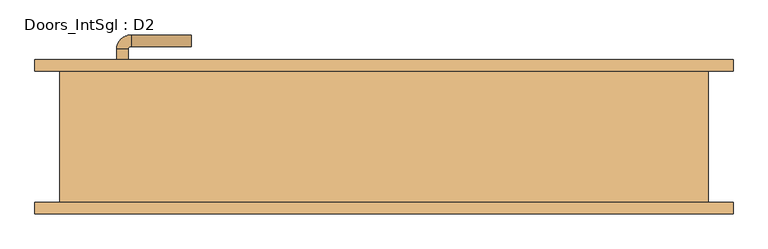
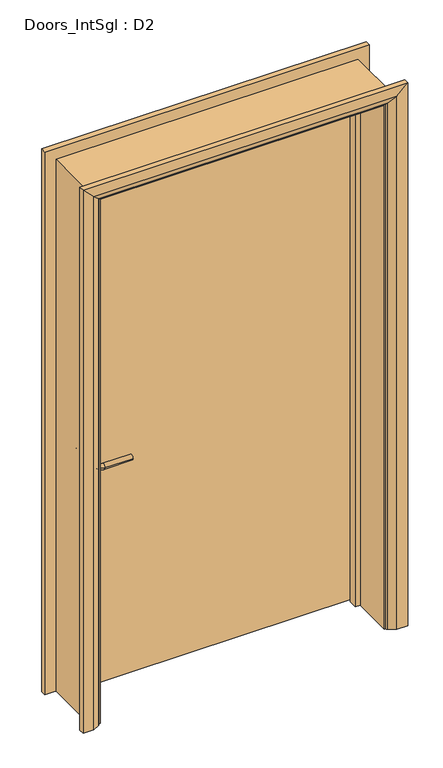
"""IFC4 building model written with IfcOpenShell, lengths in millimetres: door geometry, Doors_IntSgl : D2."""

from ifc_helpers import new_model, si_unit, point, frame, frame_2d, origin, place, context, project, spatial, polyline, circle_curve, ellipse_curve, trimmed, segment, composite_curve, outline, extrude, faceted_brep, source, transform, mapped, element, save
from ifc_brep_helpers import plane_surface, cylinder_surface, revolved_surface, advanced_brep


def doors_intsgl_d2_df50d10e(model_context):
    return source(origin(), model_context, "Body", "SolidModel", [
        advanced_brep(
        [(-464.5, 68.3, 900.0), (-444.5, 68.3, 900.0), (-444.5, 38.3, 900.0), (-464.5, 38.3, 900.0), (-439.5, 33.3, 900.0), (-439.5, 13.3, 900.0), (-334.5, 13.3, 900.0), (-334.5, 33.3, 900.0)],
        [
            (0, 1, circle_curve(frame((-454.5, 68.3, 900.0), z_axis=(0.0, 1.0, 0.0), x_axis=(1.0, 0.0, 0.0)), 10.0)),
            (1, 0, circle_curve(frame((-454.5, 68.3, 900.0), z_axis=(0.0, 1.0, 0.0), x_axis=(1.0, 0.0, 0.0)), 10.0)),
            (1, 2),
            (2, 3, circle_curve(frame((-454.5, 38.3, 900.0), z_axis=(0.0, 1.0, 0.0), x_axis=(1.0, 0.0, 0.0)), 10.0)),
            (3, 0),
            (3, 2, circle_curve(frame((-454.5, 38.3, 900.0), z_axis=(0.0, 1.0, 0.0), x_axis=(1.0, 0.0, 0.0)), 10.0)),
            (4, 5, circle_curve(frame((-439.5, 23.3, 900.0), z_axis=(-1.0, 0.0, 0.0), x_axis=(0.0, 1.0, 0.0)), 10.0)),
            (5, 3, circle_curve(frame((-439.5, 38.3, 900.0), z_axis=(0.0, 0.0, -1.0), x_axis=(-1.0, 0.0, 0.0)), 25.0)),
            (2, 4, circle_curve(frame((-439.5, 38.3, 900.0), z_axis=(0.0, 0.0, 1.0), x_axis=(-1.0, 0.0, 0.0)), 5.0)),
            (5, 4, circle_curve(frame((-439.5, 23.3, 900.0), z_axis=(-1.0, 0.0, 0.0), x_axis=(0.0, 1.0, 0.0)), 10.0)),
            (6, 7, circle_curve(frame((-334.5, 23.3, 900.0), z_axis=(1.0, 0.0, 0.0), x_axis=(0.0, 1.0, 0.0)), 10.0)),
            (7, 6, circle_curve(frame((-334.5, 23.3, 900.0), z_axis=(1.0, 0.0, 0.0), x_axis=(0.0, 1.0, 0.0)), 10.0)),
            (4, 7),
            (6, 5),
        ],
        [
            plane_surface(frame((-454.5, 68.3, 900.0), z_axis=(0.0, 1.0, 0.0), x_axis=(0.0, 0.0, 1.0))),
            cylinder_surface(frame((-454.5, 68.3, 900.0), z_axis=(0.0, 1.0, 0.0), x_axis=(1.0, 0.0, 0.0)), 10.0),
            revolved_surface(trimmed(ellipse_curve(frame((-454.5, 38.3, 900.0), z_axis=(0.0, -1.0, 0.0), x_axis=(1.0, 0.0, 0.0)), 10.0, 10.0), [point((-464.5, 38.3, 900.0))], [point((-444.5, 38.3, 900.0))], True, "CARTESIAN"), (-439.5, 38.3, 900.0), (0.0, 0.0, -1.0)),
            revolved_surface(trimmed(ellipse_curve(frame((-454.5, 38.3, 900.0), z_axis=(0.0, -1.0, 0.0), x_axis=(1.0, 0.0, 0.0)), 10.0, 10.0), [point((-444.5, 38.3, 900.0))], [point((-464.5, 38.3, 900.0))], True, "CARTESIAN"), (-439.5, 38.3, 900.0), (0.0, 0.0, -1.0)),
            plane_surface(frame((-334.5, 23.3, 900.0), z_axis=(1.0, 0.0, 0.0), x_axis=(0.0, 0.0, 1.0))),
            cylinder_surface(frame((-439.5, 23.3, 900.0), z_axis=(-1.0, 0.0, 0.0), x_axis=(0.0, 1.0, 0.0)), 10.0),
        ],
        [
            (0, [[1, 2]]),
            (1, [[3, 4, 5, -2]]),
            (1, [[-5, 6, -3, -1]]),
            (2, [[7, 8, -4, 9]]),
            (3, [[10, -9, -6, -8]]),
            (4, [[11, 12]]),
            (5, [[13, -11, 14, -7]]),
            (5, [[-14, -12, -13, -10]]),
        ],
    ),
        extrude(outline(composite_curve([segment(trimmed(circle_curve(frame_2d((900.0, -457.0)), 30.0), [point((900.0, -487.0))], [point((900.0, -427.0))], False, "CARTESIAN"), True, "CONTINUOUS"), segment(trimmed(circle_curve(frame_2d((900.0, -457.0)), 30.0), [point((900.0, -427.0))], [point((900.0, -487.0))], False, "CARTESIAN"), True, "CONTINUOUS")], self_intersect=False)), frame((0.0, 68.3, 0.0), z_axis=(0.0, 1.0, 0.0), x_axis=(0.0, 0.0, 1.0)), (0.0, 0.0, 1.0), 8.0),
        advanced_brep(
        [(-464.5, 122.3, 900.0), (-444.5, 122.3, 900.0), (-464.5, 152.3, 900.0), (-444.5, 152.3, 900.0), (-439.5, 157.3, 900.0), (-439.5, 177.3, 900.0), (-334.5, 177.3, 900.0), (-334.5, 157.3, 900.0)],
        [
            (0, 1, circle_curve(frame((-454.5, 122.3, 900.0), z_axis=(0.0, -1.0, 0.0), x_axis=(1.0, 0.0, 0.0)), 10.0)),
            (1, 0, circle_curve(frame((-454.5, 122.3, 900.0), z_axis=(0.0, -1.0, 0.0), x_axis=(1.0, 0.0, 0.0)), 10.0)),
            (0, 2),
            (2, 3, circle_curve(frame((-454.5, 152.3, 900.0), z_axis=(0.0, -1.0, 0.0), x_axis=(1.0, 0.0, 0.0)), 10.0)),
            (3, 1),
            (3, 2, circle_curve(frame((-454.5, 152.3, 900.0), z_axis=(0.0, -1.0, 0.0), x_axis=(1.0, 0.0, 0.0)), 10.0)),
            (4, 3, circle_curve(frame((-439.5, 152.3, 900.0), z_axis=(0.0, 0.0, 1.0), x_axis=(-1.0, 0.0, 0.0)), 5.0)),
            (2, 5, circle_curve(frame((-439.5, 152.3, 900.0), z_axis=(0.0, 0.0, -1.0), x_axis=(-1.0, 0.0, 0.0)), 25.0)),
            (5, 4, circle_curve(frame((-439.5, 167.3, 900.0), z_axis=(-1.0, 0.0, 0.0), x_axis=(0.0, -1.0, 0.0)), 10.0)),
            (4, 5, circle_curve(frame((-439.5, 167.3, 900.0), z_axis=(-1.0, 0.0, 0.0), x_axis=(0.0, -1.0, 0.0)), 10.0)),
            (6, 7, circle_curve(frame((-334.5, 167.3, 900.0), z_axis=(1.0, 0.0, 0.0), x_axis=(0.0, -1.0, 0.0)), 10.0)),
            (7, 6, circle_curve(frame((-334.5, 167.3, 900.0), z_axis=(1.0, 0.0, 0.0), x_axis=(0.0, -1.0, 0.0)), 10.0)),
            (5, 6),
            (7, 4),
        ],
        [
            plane_surface(frame((-454.5, 122.3, 900.0), z_axis=(0.0, -1.0, 0.0), x_axis=(0.0, 0.0, 1.0))),
            cylinder_surface(frame((-454.5, 122.3, 900.0), z_axis=(0.0, -1.0, 0.0), x_axis=(1.0, 0.0, 0.0)), 10.0),
            revolved_surface(trimmed(ellipse_curve(frame((-454.5, 152.3, 900.0), z_axis=(0.0, -1.0, 0.0), x_axis=(1.0, 0.0, 0.0)), 10.0, 10.0), [point((-464.5, 152.3, 900.0))], [point((-444.5, 152.3, 900.0))], True, "CARTESIAN"), (-439.5, 152.3, 900.0), (0.0, 0.0, -1.0)),
            revolved_surface(trimmed(ellipse_curve(frame((-454.5, 152.3, 900.0), z_axis=(0.0, -1.0, 0.0), x_axis=(1.0, 0.0, 0.0)), 10.0, 10.0), [point((-444.5, 152.3, 900.0))], [point((-464.5, 152.3, 900.0))], True, "CARTESIAN"), (-439.5, 152.3, 900.0), (0.0, 0.0, -1.0)),
            plane_surface(frame((-334.5, 167.3, 900.0), z_axis=(1.0, 0.0, 0.0), x_axis=(0.0, 0.0, 1.0))),
            cylinder_surface(frame((-439.5, 167.3, 900.0), z_axis=(-1.0, 0.0, 0.0), x_axis=(0.0, -1.0, 0.0)), 10.0),
        ],
        [
            (0, [[1, 2]]),
            (1, [[-1, 3, 4, 5]]),
            (1, [[-2, -5, 6, -3]]),
            (2, [[7, -4, 8, 9]]),
            (3, [[-8, -6, -7, 10]]),
            (4, [[11, 12]]),
            (5, [[-9, 13, -12, 14]]),
            (5, [[-10, -14, -11, -13]]),
        ],
    ),
        extrude(outline(composite_curve([segment(trimmed(circle_curve(frame_2d((900.0, -457.0)), 30.0), [point((900.0, -487.0))], [point((900.0, -427.0))], False, "CARTESIAN"), True, "CONTINUOUS"), segment(trimmed(circle_curve(frame_2d((900.0, -457.0)), 30.0), [point((900.0, -427.0))], [point((900.0, -487.0))], False, "CARTESIAN"), True, "CONTINUOUS")], self_intersect=False)), frame((0.0, 114.3, 0.0), z_axis=(0.0, 1.0, 0.0), x_axis=(0.0, 0.0, 1.0)), (0.0, 0.0, 1.0), 8.0),
        extrude(outline(polyline([(529.5, 76.3), (-529.5, 76.3), (-529.5, 114.3), (529.5, 114.3), (529.5, 76.3)])), frame((0.0, 0.0, 8.0), z_axis=(0.0, 0.0, 1.0), x_axis=(1.0, 0.0, 0.0)), (0.0, 0.0, 1.0), 2060.0),
        advanced_brep(
        [(606.5, 134.3, 0.0), (606.5, 114.3, 0.0), (536.5, 114.3, 0.0), (540.5, 120.3, 0.0), (566.5, 134.3, 0.0), (606.5, 134.3, 2145.0), (606.5, 114.3, 2145.0), (-606.5, 114.3, 2145.0), (-606.5, 114.3, 0.0), (-536.5, 114.3, 0.0), (-536.5, 114.3, 2075.0), (536.5, 114.3, 2075.0), (540.5, 120.3, 2079.0), (566.5, 134.3, 2105.0), (-566.5, 134.3, 2105.0), (-566.5, 134.3, 0.0), (-606.5, 134.3, 0.0), (-606.5, 134.3, 2145.0), (-540.5, 120.3, 0.0), (-540.5, 120.3, 2079.0)],
        [
            (0, 1),
            (1, 2),
            (2, 3, circle_curve(frame((544.5, 113.3, 0.0), z_axis=(0.0, 0.0, -1.0), x_axis=(1.0, 0.0, 0.0)), 8.0622577)),
            (3, 4),
            (4, 0),
            (0, 5),
            (5, 6),
            (6, 1),
            (6, 7),
            (7, 8),
            (8, 9),
            (9, 10),
            (10, 11),
            (11, 2),
            (11, 12, ellipse_curve(frame((544.5, 113.3, 2083.0), z_axis=(0.7071067811865475, 0.0, -0.7071067811865475), x_axis=(-0.7071067811865474, 0.0, -0.7071067811865476)), 11.4017543, 8.0622577)),
            (12, 3),
            (12, 13),
            (13, 4),
            (13, 14),
            (14, 15),
            (15, 16),
            (16, 17),
            (17, 5),
            (7, 17),
            (16, 8),
            (15, 18),
            (18, 9, circle_curve(frame((-544.5, 113.3, 0.0), z_axis=(0.0, 0.0, -1.0), x_axis=(-1.0, 0.0, 0.0)), 8.0622577)),
            (19, 10, ellipse_curve(frame((-544.5, 113.3, 2083.0), z_axis=(-0.7071067811865475, 0.0, -0.7071067811865475), x_axis=(-0.7071067811865474, 0.0, 0.7071067811865476)), 11.4017543, 8.0622577)),
            (18, 19),
            (14, 19),
            (19, 12),
        ],
        [
            plane_surface(frame((536.5, 114.3, 0.0), z_axis=(0.0, 0.0, -1.0), x_axis=(0.0, -1.0, 0.0))),
            plane_surface(frame((606.5, 134.3, 0.0), z_axis=(1.0, 0.0, 0.0), x_axis=(0.0, 0.0, 1.0))),
            plane_surface(frame((606.5, 114.3, 0.0), z_axis=(0.0, -1.0, 0.0), x_axis=(0.0, 0.0, 1.0))),
            cylinder_surface(frame((544.5, 113.3, 0.0), z_axis=(0.0, 0.0, -1.0), x_axis=(1.0, 0.0, 0.0)), 8.0622577),
            plane_surface(frame((540.5, 120.3, 0.0), z_axis=(-0.4740998230350126, 0.880471099922178, 0.0), x_axis=(0.0, 0.0, 1.0))),
            plane_surface(frame((566.5, 134.3, 0.0), z_axis=(0.0, 1.0, 0.0), x_axis=(0.0, 0.0, 1.0))),
            plane_surface(frame((-606.5, 134.3, 2145.0), z_axis=(-1.0, 0.0, 0.0), x_axis=(0.0, 0.0, -1.0))),
            plane_surface(frame((-536.5, 114.3, 0.0), z_axis=(0.0, 0.0, -1.0), x_axis=(0.0, -1.0, 0.0))),
            cylinder_surface(frame((-544.5, 113.3, 2075.0), z_axis=(0.0, 0.0, 1.0), x_axis=(-1.0, 0.0, 0.0)), 8.0622577),
            plane_surface(frame((-540.5, 120.3, 2079.0), z_axis=(0.47409982303501824, 0.8804710999221749, 0.0), x_axis=(0.0, 0.0, -1.0))),
            plane_surface(frame((606.5, 134.3, 2145.0), z_axis=(0.0, 0.0, 1.0), x_axis=(-1.0, 0.0, 0.0))),
            cylinder_surface(frame((536.5, 113.3, 2083.0), z_axis=(1.0, 0.0, 0.0), x_axis=(0.0, 0.0, 1.0)), 8.0622577),
            plane_surface(frame((540.5, 120.3, 2079.0), z_axis=(0.0, 0.8804710999221764, -0.4740998230350154), x_axis=(-1.0, 0.0, 0.0))),
        ],
        [
            (0, [[1, 2, 3, 4, 5]]),
            (1, [[-1, 6, 7, 8]]),
            (2, [[-2, -8, 9, 10, 11, 12, 13, 14]]),
            (3, [[-3, -14, 15, 16]]),
            (4, [[-4, -16, 17, 18]]),
            (5, [[-5, -18, 19, 20, 21, 22, 23, -6]]),
            (6, [[24, -22, 25, -10]]),
            (7, [[-21, 26, 27, -11, -25]]),
            (8, [[28, -12, -27, 29]]),
            (9, [[30, -29, -26, -20]]),
            (10, [[-7, -23, -24, -9]]),
            (11, [[-15, -13, -28, 31]]),
            (12, [[-17, -31, -30, -19]]),
        ],
    ),
        extrude(outline(polyline([(0.0, -531.5), (0.0, -512.5), (2051.0, -512.5), (2051.0, 512.5), (0.0, 512.5), (0.0, 531.5), (2070.0, 531.5), (2070.0, -531.5), (0.0, -531.5)])), frame((0.0, 42.3, 0.0), z_axis=(0.0, 1.0, 0.0), x_axis=(0.0, 0.0, 1.0)), (0.0, 0.0, 1.0), 32.0),
        advanced_brep(
        [(-606.5, -134.3, 0.0), (-606.5, -114.3, 0.0), (-536.5, -114.3, 0.0), (-540.5, -120.3, 0.0), (-566.5, -134.3, 0.0), (-606.5, -134.3, 2145.0), (-606.5, -114.3, 2145.0), (-536.5, -114.3, 2075.0), (-540.5, -120.3, 2079.0), (-566.5, -134.3, 2105.0), (606.5, -134.3, 0.0), (566.5, -134.3, 0.0), (540.5, -120.3, 0.0), (536.5, -114.3, 0.0), (606.5, -114.3, 0.0), (606.5, -134.3, 2145.0), (566.5, -134.3, 2105.0), (540.5, -120.3, 2079.0), (536.5, -114.3, 2075.0), (606.5, -114.3, 2145.0)],
        [
            (0, 1),
            (1, 2),
            (2, 3, circle_curve(frame((-544.5, -113.3, 0.0), z_axis=(0.0, 0.0, -1.0), x_axis=(-1.0, 0.0, 0.0)), 8.0622577)),
            (3, 4),
            (4, 0),
            (0, 5),
            (5, 6),
            (6, 1),
            (6, 7),
            (7, 2),
            (7, 8, ellipse_curve(frame((-544.5, -113.3, 2083.0), z_axis=(-0.7071067811865475, 0.0, -0.7071067811865475), x_axis=(0.7071067811865474, 0.0, -0.7071067811865476)), 11.4017543, 8.0622577)),
            (8, 3),
            (8, 9),
            (9, 4),
            (9, 5),
            (10, 11),
            (11, 12),
            (12, 13, circle_curve(frame((544.5, -113.3, 0.0), z_axis=(0.0, 0.0, -1.0), x_axis=(1.0, 0.0, 0.0)), 8.0622577)),
            (13, 14),
            (14, 10),
            (15, 16),
            (16, 11),
            (10, 15),
            (16, 17),
            (17, 12),
            (17, 18, ellipse_curve(frame((544.5, -113.3, 2083.0), z_axis=(0.7071067811865475, 0.0, -0.7071067811865475), x_axis=(0.7071067811865474, 0.0, 0.7071067811865476)), 11.4017543, 8.0622577)),
            (18, 13),
            (18, 19),
            (19, 14),
            (19, 15),
            (5, 15),
            (19, 6),
            (18, 7),
            (17, 8),
            (16, 9),
        ],
        [
            plane_surface(frame((-536.5, -187.1010989, 0.0), z_axis=(0.0, 0.0, -1.0), x_axis=(1.0, 0.0, 0.0))),
            plane_surface(frame((-606.5, -134.3, 0.0), z_axis=(-1.0, 0.0, 0.0), x_axis=(0.0, 0.0, 1.0))),
            plane_surface(frame((-606.5, -114.3, 0.0), z_axis=(0.0, 1.0, 0.0), x_axis=(0.0, 0.0, 1.0))),
            cylinder_surface(frame((-544.5, -113.3, 0.0), z_axis=(0.0, 0.0, -1.0), x_axis=(-1.0, 0.0, 0.0)), 8.0622577),
            plane_surface(frame((-540.5, -120.3, 0.0), z_axis=(0.4740998230350183, -0.8804710999221749, 0.0), x_axis=(0.0, 0.0, 1.0))),
            plane_surface(frame((-566.5, -134.3, 0.0), z_axis=(0.0, -1.0, 0.0), x_axis=(0.0, 0.0, 1.0))),
            plane_surface(frame((536.5, -187.1010989, 0.0), z_axis=(0.0, 0.0, -1.0), x_axis=(-1.0, 0.0, 0.0))),
            plane_surface(frame((566.5, -134.3, 2105.0), z_axis=(0.0, -1.0, 0.0), x_axis=(0.0, 0.0, -1.0))),
            plane_surface(frame((540.5, -120.3, 2079.0), z_axis=(-0.4740998230350183, -0.8804710999221749, 0.0), x_axis=(0.0, 0.0, -1.0))),
            cylinder_surface(frame((544.5, -113.3, 2075.0), z_axis=(0.0, 0.0, 1.0), x_axis=(1.0, 0.0, 0.0)), 8.0622577),
            plane_surface(frame((606.5, -114.3, 2145.0), z_axis=(0.0, 1.0, 0.0), x_axis=(0.0, 0.0, -1.0))),
            plane_surface(frame((606.5, -134.3, 2145.0), z_axis=(1.0, 0.0, 0.0), x_axis=(0.0, 0.0, -1.0))),
            plane_surface(frame((-606.5, -134.3, 2145.0), z_axis=(0.0, 0.0, 1.0), x_axis=(1.0, 0.0, 0.0))),
            plane_surface(frame((-606.5, -114.3, 2145.0), z_axis=(0.0, 1.0, 0.0), x_axis=(1.0, 0.0, 0.0))),
            cylinder_surface(frame((-536.5, -113.3, 2083.0), z_axis=(-1.0, 0.0, 0.0), x_axis=(0.0, 0.0, 1.0)), 8.0622577),
            plane_surface(frame((-540.5, -120.3, 2079.0), z_axis=(0.0, -0.8804710999221749, -0.4740998230350183), x_axis=(1.0, 0.0, 0.0))),
            plane_surface(frame((-566.5, -134.3, 2105.0), z_axis=(0.0, -1.0, 0.0), x_axis=(1.0, 0.0, 0.0))),
        ],
        [
            (0, [[1, 2, 3, 4, 5]]),
            (1, [[-1, 6, 7, 8]]),
            (2, [[-2, -8, 9, 10]]),
            (3, [[-3, -10, 11, 12]]),
            (4, [[-4, -12, 13, 14]]),
            (5, [[-5, -14, 15, -6]]),
            (6, [[16, 17, 18, 19, 20]]),
            (7, [[21, 22, -16, 23]]),
            (8, [[24, 25, -17, -22]]),
            (9, [[26, 27, -18, -25]]),
            (10, [[28, 29, -19, -27]]),
            (11, [[30, -23, -20, -29]]),
            (12, [[-7, 31, -30, 32]]),
            (13, [[-9, -32, -28, 33]]),
            (14, [[-11, -33, -26, 34]]),
            (15, [[-13, -34, -24, 35]]),
            (16, [[-15, -35, -21, -31]]),
        ],
    ),
        faceted_brep([(-531.5, 114.3, 0.0), (-531.5, -114.3, 0.0), (-563.5, -114.3, 0.0), (-563.5, 114.3, 0.0), (-531.5, 114.3, 2070.0), (-531.5, -114.3, 2070.0), (-563.5, -114.3, 2102.0), (-563.5, 114.3, 2102.0), (531.5, 114.3, 0.0), (563.5, 114.3, 0.0), (563.5, -114.3, 0.0), (531.5, -114.3, 0.0), (531.5, 114.3, 2070.0), (563.5, 114.3, 2102.0), (563.5, -114.3, 2102.0), (531.5, -114.3, 2070.0)], [[[0, 1, 2, 3]], [[1, 0, 4, 5]], [[2, 1, 5, 6]], [[3, 2, 6, 7]], [[0, 3, 7, 4]], [[8, 9, 10, 11]], [[12, 13, 9, 8]], [[13, 14, 10, 9]], [[14, 15, 11, 10]], [[15, 12, 8, 11]], [[5, 4, 12, 15]], [[6, 5, 15, 14]], [[7, 6, 14, 13]], [[4, 7, 13, 12]]]),
    ])


if __name__ == "__main__":
    model = new_model("IFC4")
    model_context = context("Model", 3, world=origin())
    ifc_project = project(units=[si_unit("LENGTHUNIT", "METRE", prefix="MILLI")], contexts=[model_context])
    site = spatial("IfcSite", under=ifc_project)
    building = spatial("IfcBuilding", under=site)
    placement = place(None, origin())
    doors_intsgl_d2_shape = doors_intsgl_d2_df50d10e(model_context)
    element("IfcDoor", 1, ObjectType="Doors_IntSgl : D2", at=placement, inside=building, context=model_context, shape_type="MappedRepresentation", body=[
        mapped(doors_intsgl_d2_shape, transform((0.0, 0.0, 0.0), x_axis=(1.0, 0.0, 0.0), y_axis=(0.0, 1.0, 0.0), z_axis=(0.0, 0.0, 1.0))),
    ])
    save(model, "model.ifc")

# Revit data of these elements
# Type "Doors_IntSgl : D2"
#   Type Mark = "47"
#   Type Comments = "Internal Single"
#   Operation = "SingleSwingRight"
#   Manufacturer = "Revit"
#   Keynote = "L20"
#   Description = "Internal Single Door"
#   Analytic Construction = "Metal"
#   UnderCut = 8 mm
#   Tolerance = 2 mm
#   Thickness = 38 mm
#   Thermal Resistance (R) = 0.270117 (m²·K)/W
#   Structural Tolerance = 8 mm
#   StopDepth = 32 mm
#   Stop Thickness = 19 mm
#   Rough Width = 1143 mm
#   Rough Height = 2110 mm
#   Height to Top Lock Rail = 1000 mm
#   Heat Transfer Coefficient (U) = 3.7021 W/(m²·K)
#   Handle Z Distance = 900 mm
#   Handle X Distance = 75 mm
#   Frame Thickness = 32 mm
#   Door Panel Width = 1059 mm
#   Door Panel Thickness = 38 mm
#   Door Panel Offset = 0 mm
#   Height = 2110 mm
#   Width = 1143 mm
#   Door Panel Height = 2060 mm
#   Architrave Setback = 5 mm
#   Vis - Ironmongery = yes
#   Material Ironmongery = Door - Handle
#   Material Frame = Door - Frame/Mullion (1)
#   Material Door = Door - Panel
#   Material Architrave = Door - Architrave
#   Visual Light Transmittance = 0
#   Solar Heat Gain Coefficient = 0
#   Function = (empty or 0)
#   Wall Closure = (empty or 0)
# Element 1 (IfcDoor, "Doors_IntSgl : D2")
#   Materials on its faces: "Door - Architrave", "Door - Handle", "Door - Frame/Mullion (1)", "Door - Panel"
# Materials
#   "Door - Handle": colour RGB 0 0 0, transparency 0, Keynote = "P21", Cost = 0
#   "Door - Frame/Mullion (1)": class "Wood", colour RGB 212 179 113, transparency 0, Keynote = "L20", Cost = 0
#   "Door - Panel": class "Wood", colour RGB 210 159 95, transparency 0, Keynote = "L20", Cost = 0
#   "Door - Architrave": class "Wood", colour RGB 154 90 5, transparency 0, Keynote = "P20", Cost = 0
